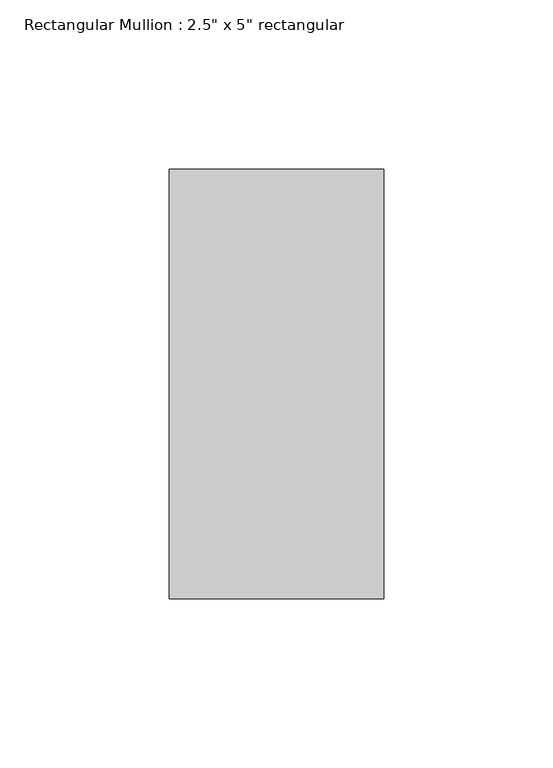
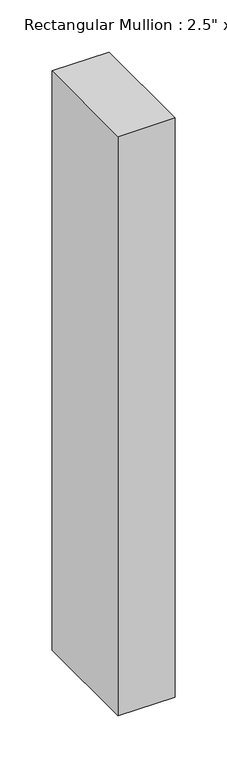
"""IFC4 building model written with IfcOpenShell, lengths in millimetres: member geometry."""

from ifc_helpers import new_model, si_unit, frame, origin, place, context, project, spatial, polyline, outline, extrude, source, transform, mapped, element, save


def member_3cbf331d(model_context):
    return source(origin(), model_context, "Body", "SweptSolid", [
        extrude(outline(polyline([(0.0, 63.5), (0.0, -63.5), (-63.5, -63.5), (-63.5, 63.5), (0.0, 63.5)])), frame((0.0, 0.0, -679.4500043), z_axis=(0.0, 0.0, 1.0), x_axis=(1.0, 0.0, 0.0)), (0.0, 0.0, 1.0), 679.4500043),
    ])


if __name__ == "__main__":
    model = new_model("IFC4")
    model_context = context("Model", 3, world=origin())
    ifc_project = project(units=[si_unit("LENGTHUNIT", "METRE", prefix="MILLI")], contexts=[model_context])
    site = spatial("IfcSite", under=ifc_project)
    building = spatial("IfcBuilding", under=site)
    placement = place(None, origin())
    member_shape = member_3cbf331d(model_context)
    element("IfcMember", 1, ObjectType="Rectangular Mullion : 2.5\" x 5\" rectangular", at=placement, inside=building, context=model_context, shape_type="MappedRepresentation", body=[
        mapped(member_shape, transform((0.0, 0.0, 0.0), x_axis=(1.0, 0.0, 0.0), y_axis=(0.0, 1.0, 0.0), z_axis=(0.0, 0.0, 1.0))),
    ])
    save(model, "model.ifc")

# Revit data of these elements
# Type "Rectangular Mullion : 2.5\" x 5\" rectangular"
#   built-in parameter 1007304 = 0.416667 (stored number, unit not read)
#   built-in parameter 1007301 = 0.104167 (stored number, unit not read)
#   built-in parameter 1007300 = 0.104167 (stored number, unit not read)
# Element 1 (IfcMember, "Rectangular Mullion : 2.5\" x 5\" rectangular")
#   Materials on its faces: "Aluminum"
# Materials
#   "Aluminum": class "Metal", colour RGB 247 247 247, transparency 0, Description = "Aluminum 6061", Cost = 0
